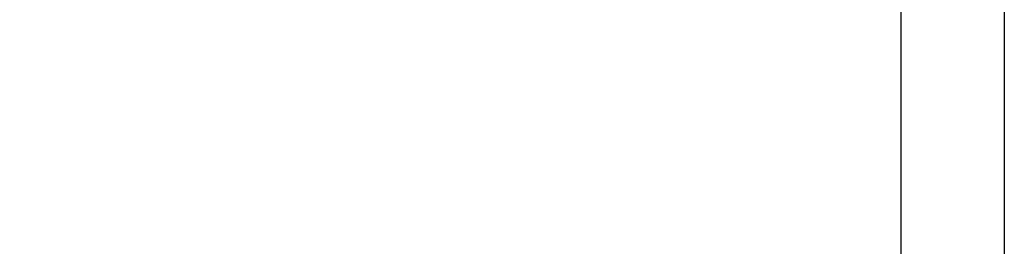
# Model space of a CAD drawing. Units: inches. Extents: x 2091 to 2899, y 967 to 2217.
# Tile 32 of 256: x 2390 to 2459, y 1065 to 1081. Entities that reach past the tile are written whole.
import ezdxf

# ---------------------------------------------------------------- set-up
doc = ezdxf.new("R2010")
doc.units = ezdxf.units.IN
doc.layers.add('A-ANNO-DIMS', color=2, linetype='Continuous', lineweight=18)
doc.styles.get("Standard").update_dxf_attribs({"font": 'arial.ttf'})
doc.dimstyles.new('ISO-25', dxfattribs={"dimtxt": 4, "dimasz": 4, "dimexe": 1.25, "dimexo": 0.625, "dimtad": 1, "dimdec": 0, "dimlunit": 3, "dimtxsty": 'Standard', "dimcen": 2.5, "dimadec": 0, "dimazin": 0, "dimtfac": 1, "dimtdec": 0, "dimtmove": 0, "dimatfit": 3, "dimfxl": 1, "dimarcsym": 0})

# ---------------------------------------------------------------- blocks, each defined once
blk = doc.blocks.new('*D68')
at = {"layer": 'A-ANNO-DIMS', "color": 0, "lineweight": -2, "transparency": 16777216}
for p, q in [((2317.144, 1535.794), (2317.144, 969.464)), ((2459.384, 1535.794), (2459.384, 969.464)), ((2321.144, 970.714), (2455.384, 970.714))]:
    blk.add_line(p, q, dxfattribs=at)
at = {"layer": 'A-ANNO-DIMS', "color": 0, "transparency": 16777216}
for points in [[(2321.144, 971.381), (2321.144, 970.048), (2317.144, 970.714)], [(2455.384, 971.381), (2455.384, 970.048), (2459.384, 970.714)]]:
    blk.add_solid(points, dxfattribs=at)
at = {"layer": 'Defpoints', "color": 0, "transparency": 16777216}
for p in [(2317.144, 1536.419), (2459.384, 1536.419), (2459.384, 970.714)]:
    blk.add_point(p, dxfattribs=at)
at = {"layer": 'A-ANNO-DIMS', "color": 0, "transparency": 16777216, "insert": (2388.264, 973.382), "char_height": 4, "attachment_point": 5}
blk.add_mtext('11\'-10"', dxfattribs=at)
blk = doc.blocks.new('*D71')
at = {"layer": 'A-ANNO-DIMS', "color": 0, "lineweight": -2, "transparency": 16777216}
for p, q in [((2212.144, 1351.294), (2212.144, 969.464)), ((2452.144, 1351.294), (2452.144, 969.464)), ((2216.144, 970.714), (2448.144, 970.714))]:
    blk.add_line(p, q, dxfattribs=at)
at = {"layer": 'A-ANNO-DIMS', "color": 0, "transparency": 16777216}
for points in [[(2216.144, 971.381), (2216.144, 970.048), (2212.144, 970.714)], [(2448.144, 971.381), (2448.144, 970.048), (2452.144, 970.714)]]:
    blk.add_solid(points, dxfattribs=at)
at = {"layer": 'Defpoints', "color": 0, "transparency": 16777216}
for p in [(2212.144, 1351.919), (2452.144, 1351.919), (2452.144, 970.714)]:
    blk.add_point(p, dxfattribs=at)
at = {"layer": 'A-ANNO-DIMS', "color": 0, "transparency": 16777216, "insert": (2332.144, 973.382), "char_height": 4, "attachment_point": 5}
blk.add_mtext('20\'-0"', dxfattribs=at)

msp = doc.modelspace()

# ---------------------------------------------------------------- dimensions: what is measured, and where the dimension line sits
at = {"layer": 'A-ANNO-DIMS'}
for base, p1, p2, picture, middle in [((2459.384, 970.714), (2317.144, 1536.419), (2459.384, 1536.419), '*D68', (2388.264, 973.382)), ((2452.144, 970.714), (2212.144, 1351.919), (2452.144, 1351.919), '*D71', (2332.144, 973.382))]:
    dim = msp.add_linear_dim(base=base, p1=p1, p2=p2, dimstyle='ISO-25', override={"dimdec": 1, "dimlfac": 1, "dimrnd": 0, "dimzin": 1, "dimdsep": 46, "dimlunit": 4, "dimfrac": 2}, dxfattribs=at)
    dim.commit()
    dim.dimension.update_dxf_attribs({"geometry": picture, "text_midpoint": middle})

doc.saveas('drawing.dxf')
